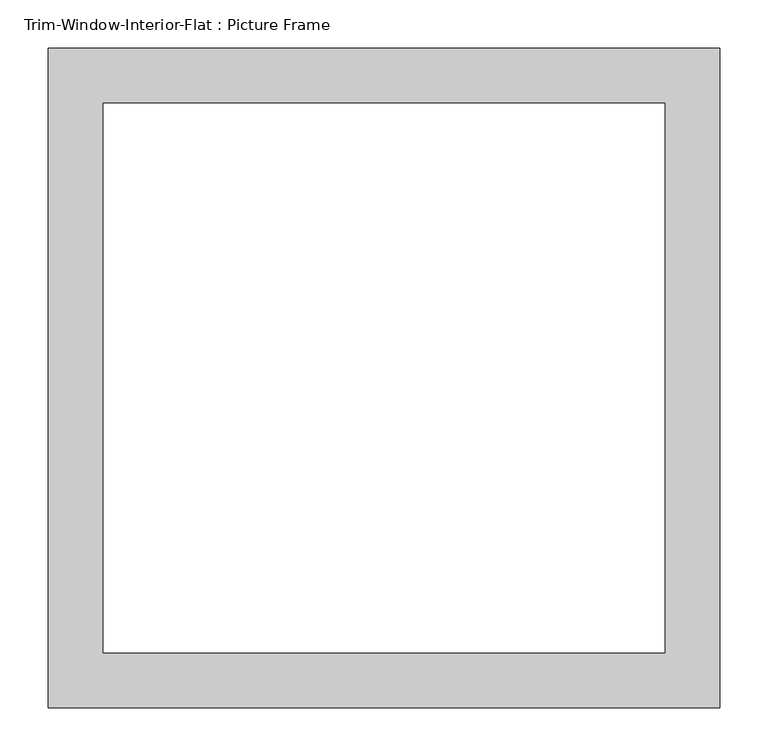
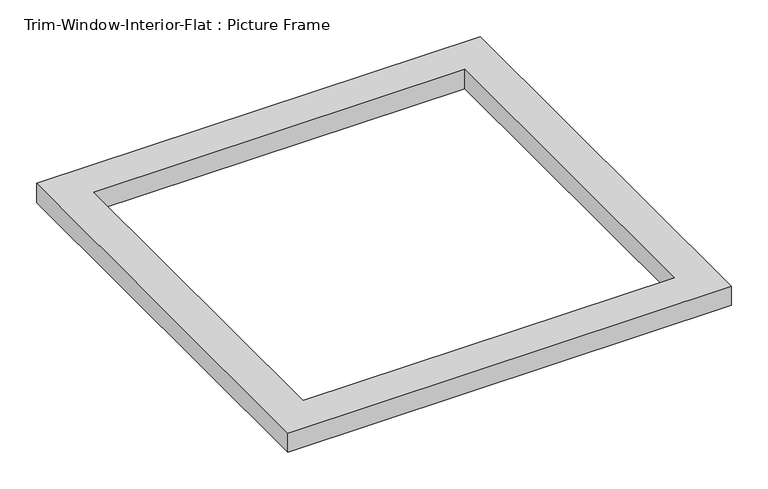
"""IFC4 building model written with IfcOpenShell, lengths in millimetres: proxy geometry, Trim-Window-Interior-Flat : Picture Frame."""

from ifc_helpers import new_model, si_unit, origin, origin_with_axes, place, context, project, spatial, polyline, outline, extrude, source, transform, mapped, element, save


def trim_window_interior_flat_picture_frame_0477b583(model_context):
    return source(origin(), model_context, "Body", "SweptSolid", [
        extrude(outline(polyline([(349.25, 44.45), (349.25, -641.35), (-349.25, -641.35), (-349.25, 44.45), (349.25, 44.45)]), holes=[polyline([(292.1, -12.7), (-292.1, -12.7), (-292.1, -584.2), (292.1, -584.2), (292.1, -12.7)])]), origin_with_axes(), (0.0, 0.0, 1.0), 31.75),
    ])


if __name__ == "__main__":
    model = new_model("IFC4")
    model_context = context("Model", 3, world=origin())
    ifc_project = project(units=[si_unit("LENGTHUNIT", "METRE", prefix="MILLI")], contexts=[model_context])
    site = spatial("IfcSite", under=ifc_project)
    building = spatial("IfcBuilding", under=site)
    placement = place(None, origin())
    trim_window_interior_flat_picture_frame_shape = trim_window_interior_flat_picture_frame_0477b583(model_context)
    element("IfcBuildingElementProxy", 1, Name="Trim-Window-Interior-Flat : Picture Frame", ObjectType="Trim-Window-Interior-Flat : Picture Frame", at=placement, inside=building, context=model_context, shape_type="MappedRepresentation", body=[
        mapped(trim_window_interior_flat_picture_frame_shape, transform((0.0, 0.0, 0.0), x_axis=(1.0, 0.0, 0.0), y_axis=(0.0, 1.0, 0.0), z_axis=(0.0, 0.0, 1.0))),
    ])
    save(model, "model.ifc")

# Revit data of these elements
# Type "Trim-Window-Interior-Flat : Picture Frame"
#   Trim Thickness_Picture Frame = 0' - 1 1/4"
#   Trim Width = 0' - 2 1/4"
#   Trim Thickness_with Sill = 0' - 0 3/4"
#   Sill Thickness = 0' - 1 1/4"
#   Opening Width [instance default] = 2' - 0"
#   Opening Height [instance default] = 3' - 0"
#   Default Elevation = 4' - 0"
#   Sill = no
#   Picture Frame = yes
#   Trim Material [instance default] = none
# Element 1 (IfcBuildingElementProxy, "Trim-Window-Interior-Flat : Picture Frame")
#   Opening Height = 1' - 11 1/2"
#   Trim Material = Wood - Stained
#   Materials on its faces: "Wood - Stained"
# Materials
#   "Wood - Stained": class "Wood", colour RGB 224 178 126, transparency 0, Cost = 0
